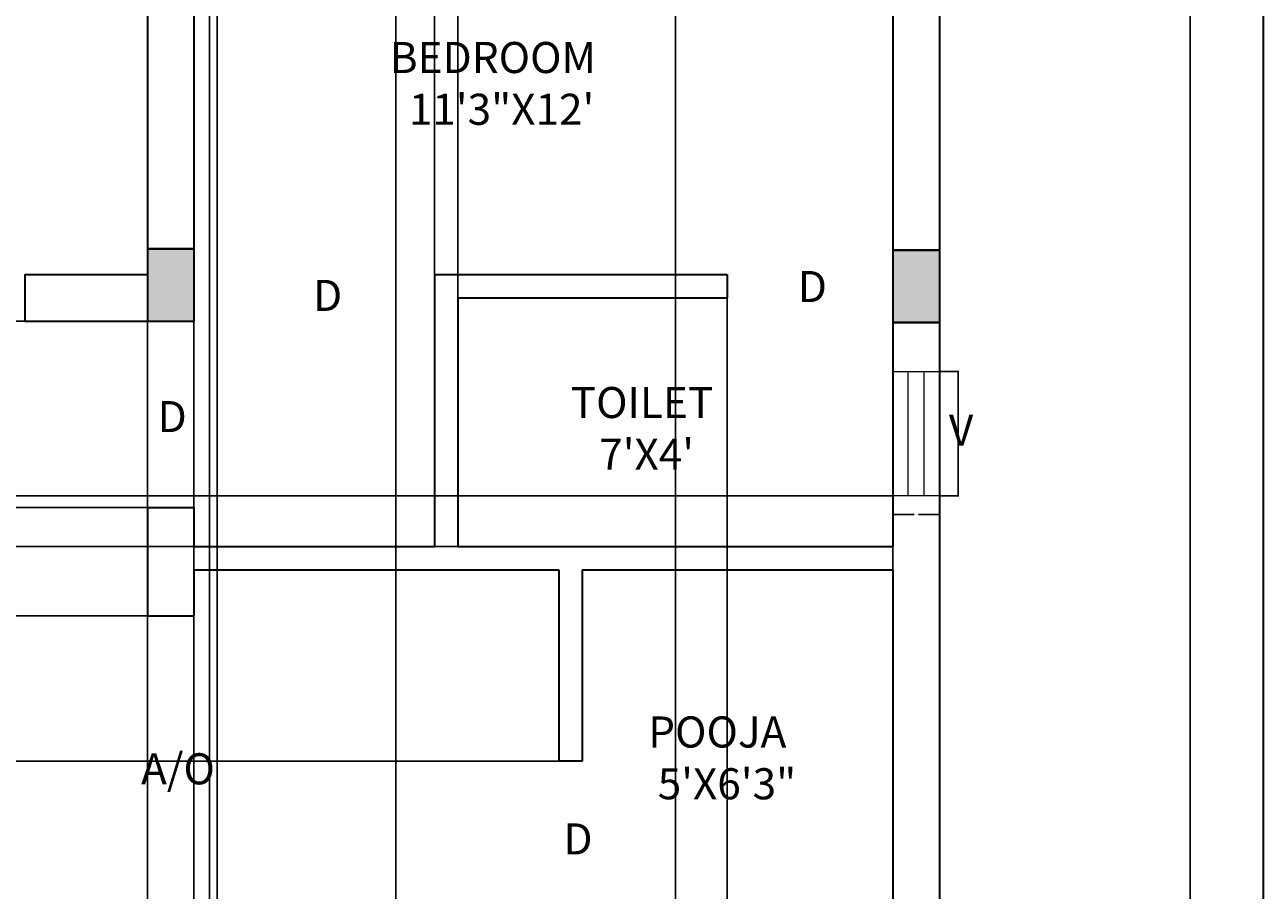
# Model space of a CAD drawing. Units: inches. Extents: x 2243 to 2668, y 14541 to 15226.
# Tile 4 of 5: x 2428 to 2668, y 14904 to 15071. Entities that reach past the tile are written whole.
import ezdxf

# ---------------------------------------------------------------- set-up
doc = ezdxf.new("R2010")
doc.units = ezdxf.units.IN
doc.header["$MEASUREMENT"] = 0
for name, color, linetype, lineweight in [('A-ANNO-DIMS', 2, 'Continuous', 18), ('A-ANNO-SYMB', 3, 'Continuous', 18), ('A-ANNO-TTLB', 7, 'Continuous', 35), ('A-AREA-IDEN', 7, 'Continuous', 18), ('A-COLS', 7, 'Continuous', 40), ('A-COLS-PATT', 7, 'Continuous', 13), ('A-GLAZ-VENT', 4, 'Continuous', 18), ('A-WALL', 7, 'Continuous', 35)]:
    doc.layers.add(name, color=color, linetype=linetype, lineweight=lineweight)
doc.styles.get("Standard").update_dxf_attribs({"font": 'arial.ttf'})
doc.dimstyles.get("Standard").update_dxf_attribs({"dimtxt": 0.18, "dimasz": 0.18, "dimexe": 0.18, "dimexo": 0.0625, "dimgap": 0.09, "dimtad": 0, "dimtih": 1, "dimtoh": 1, "dimdec": 4, "dimzin": 0, "dimdsep": 46, "dimtxsty": 'Standard', "dimcen": 0.09, "dimadec": 0, "dimazin": 0, "dimtfac": 1, "dimtdec": 4, "dimtofl": 0, "dimtmove": 0, "dimatfit": 3, "dimfxl": 1, "dimtolj": 1, "dimtzin": 0, "dimarcsym": 0})

# ---------------------------------------------------------------- blocks, each defined once
blk = doc.blocks.new('VENT-24IN')
for p, q in [((0, 24), (9, 24)), ((0, 0), (0, 24)), ((3, 0), (3, 24)), ((6, 24), (6, 0)), ((9, 24), (9, 0)), ((9, 0), (0, 0))]:
    blk.add_line(p, q)
blk = doc.blocks.new('*D9')
at = {"layer": 'A-ANNO-DIMS', "color": 0, "lineweight": -2, "transparency": 16777216}
for p, q in [((2605.02, 15004.42), (2608.74, 15004.42)), ((2608.56, 15004.24), (2608.56, 14992.6)), ((2608.56, 14980.6), (2608.56, 14992.24)), ((2605.02, 14980.42), (2608.74, 14980.42))]:
    blk.add_line(p, q, dxfattribs=at)
at = {"layer": 'A-ANNO-DIMS', "color": 0, "transparency": 16777216}
for points in [[(2608.53, 15004.24), (2608.59, 15004.24), (2608.56, 15004.42)], [(2608.53, 14980.6), (2608.59, 14980.6), (2608.56, 14980.42)]]:
    blk.add_solid(points, dxfattribs=at)
at = {"layer": 'Defpoints', "color": 0, "transparency": 16777216}
for p in [(2604.96, 15004.42), (2608.56, 15004.42), (2604.96, 14980.42)]:
    blk.add_point(p, dxfattribs=at)
at = {"layer": 'A-ANNO-DIMS', "color": 0, "transparency": 16777216, "insert": (2608.56, 14992.42), "char_height": 0.18, "attachment_point": 5}
blk.add_mtext('\\A1;VENT 24 TYP.', dxfattribs=at)
blk = doc.blocks.new('*D10')
at = {"layer": 'A-ANNO-DIMS', "color": 0, "lineweight": -2, "transparency": 16777216}
for p, q in [((2595.96, 14980.35), (2595.96, 14976.64)), ((2604.96, 14980.35), (2604.96, 14976.64)), ((2596.14, 14976.82), (2600, 14976.82)), ((2604.78, 14976.82), (2600.92, 14976.82))]:
    blk.add_line(p, q, dxfattribs=at)
at = {"layer": 'A-ANNO-DIMS', "color": 0, "transparency": 16777216}
for points in [[(2596.14, 14976.85), (2596.14, 14976.79), (2595.96, 14976.82)], [(2604.78, 14976.85), (2604.78, 14976.79), (2604.96, 14976.82)]]:
    blk.add_solid(points, dxfattribs=at)
at = {"layer": 'Defpoints', "color": 0, "transparency": 16777216}
for p in [(2595.96, 14980.42), (2604.96, 14980.42), (2604.96, 14976.82)]:
    blk.add_point(p, dxfattribs=at)
at = {"layer": 'A-ANNO-DIMS', "color": 0, "transparency": 16777216, "insert": (2600.46, 14976.82), "char_height": 0.18, "attachment_point": 5}
blk.add_mtext('\\A1;9 TYP.', dxfattribs=at)
blk = doc.blocks.new('*D18')
at = {"layer": 'A-ANNO-DIMS', "color": 0, "lineweight": -2, "transparency": 16777216}
for p, q in [((2605.02, 15176.14), (2653.58, 15176.14)), ((2653.4, 15175.96), (2653.4, 14877.07)), ((2653.4, 14577.82), (2653.4, 14876.7)), ((2605.02, 14577.64), (2653.58, 14577.64))]:
    blk.add_line(p, q, dxfattribs=at)
at = {"layer": 'A-ANNO-DIMS', "color": 0, "transparency": 16777216}
for points in [[(2653.37, 15175.96), (2653.43, 15175.96), (2653.4, 15176.14)], [(2653.37, 14577.82), (2653.43, 14577.82), (2653.4, 14577.64)]]:
    blk.add_solid(points, dxfattribs=at)
at = {"layer": 'Defpoints', "color": 0, "transparency": 16777216}
for p in [(2604.96, 15176.14), (2653.4, 15176.14), (2604.96, 14577.64)]:
    blk.add_point(p, dxfattribs=at)
at = {"layer": 'A-ANNO-DIMS', "color": 0, "transparency": 16777216, "insert": (2653.4, 14876.89), "char_height": 0.18, "attachment_point": 5}
blk.add_mtext('\\A1;598.5', dxfattribs=at)
blk = doc.blocks.new('*D31')
at = {"layer": 'A-ANNO-DIMS', "color": 0, "lineweight": -2, "transparency": 16777216}
for p, q in [((2595.9, 14980.42), (2243.57, 14980.42)), ((2243.75, 14980.24), (2243.75, 14975.71)), ((2243.75, 14970.82), (2243.75, 14975.34)), ((2595.9, 14970.64), (2243.57, 14970.64))]:
    blk.add_line(p, q, dxfattribs=at)
at = {"layer": 'A-ANNO-DIMS', "color": 0, "transparency": 16777216}
for points in [[(2243.72, 14980.24), (2243.78, 14980.24), (2243.75, 14980.42)], [(2243.72, 14970.82), (2243.78, 14970.82), (2243.75, 14970.64)]]:
    blk.add_solid(points, dxfattribs=at)
at = {"layer": 'Defpoints', "color": 0, "transparency": 16777216}
for p in [(2243.75, 14980.42), (2595.96, 14980.42), (2595.96, 14970.64)]:
    blk.add_point(p, dxfattribs=at)
at = {"layer": 'A-ANNO-DIMS', "color": 0, "transparency": 16777216, "insert": (2243.75, 14975.53), "char_height": 0.18, "attachment_point": 5}
blk.add_mtext('\\A1;9.78', dxfattribs=at)
blk = doc.blocks.new('*D35')
at = {"layer": 'A-ANNO-DIMS', "color": 0, "lineweight": -2, "transparency": 16777216}
for p, q in [((2411.89, 14673.7), (2411.89, 15225.04)), ((2412.07, 15224.86), (2431.53, 15224.86)), ((2451.78, 15224.86), (2432.32, 15224.86)), ((2451.96, 14673.7), (2451.96, 15225.04))]:
    blk.add_line(p, q, dxfattribs=at)
at = {"layer": 'A-ANNO-DIMS', "color": 0, "transparency": 16777216}
for points in [[(2412.07, 15224.89), (2412.07, 15224.83), (2411.89, 15224.86)], [(2451.78, 15224.89), (2451.78, 15224.83), (2451.96, 15224.86)]]:
    blk.add_solid(points, dxfattribs=at)
at = {"layer": 'Defpoints', "color": 0, "transparency": 16777216}
for p in [(2451.96, 15224.86), (2411.89, 14673.64), (2451.96, 14673.64)]:
    blk.add_point(p, dxfattribs=at)
at = {"layer": 'A-ANNO-DIMS', "color": 0, "transparency": 16777216, "insert": (2431.93, 15224.86), "char_height": 0.18, "attachment_point": 5}
blk.add_mtext('\\A1;40.07', dxfattribs=at)
blk = doc.blocks.new('*D36')
at = {"layer": 'A-ANNO-DIMS', "color": 0, "lineweight": -2, "transparency": 16777216}
for p, q in [((2460.96, 14673.7), (2460.96, 15225.04)), ((2461.14, 15224.86), (2462.95, 15224.86)), ((2465.28, 15224.86), (2463.47, 15224.86)), ((2465.46, 14673.7), (2465.46, 15225.04))]:
    blk.add_line(p, q, dxfattribs=at)
at = {"layer": 'A-ANNO-DIMS', "color": 0, "transparency": 16777216}
for points in [[(2461.14, 15224.89), (2461.14, 15224.83), (2460.96, 15224.86)], [(2465.28, 15224.89), (2465.28, 15224.83), (2465.46, 15224.86)]]:
    blk.add_solid(points, dxfattribs=at)
at = {"layer": 'Defpoints', "color": 0, "transparency": 16777216}
for p in [(2465.46, 15224.86), (2460.96, 14673.64), (2465.46, 14673.64)]:
    blk.add_point(p, dxfattribs=at)
at = {"layer": 'A-ANNO-DIMS', "color": 0, "transparency": 16777216, "insert": (2463.21, 15224.86), "char_height": 0.18, "attachment_point": 5}
blk.add_mtext('\\A1;4.5', dxfattribs=at)
blk = doc.blocks.new('*D37')
at = {"layer": 'A-ANNO-DIMS', "color": 0, "lineweight": -2, "transparency": 16777216}
for p, q in [((2463.96, 14586.7), (2463.96, 15225.04)), ((2464.14, 15224.86), (2508.74, 15224.86)), ((2553.78, 15224.86), (2509.18, 15224.86)), ((2553.96, 14586.7), (2553.96, 15225.04))]:
    blk.add_line(p, q, dxfattribs=at)
at = {"layer": 'A-ANNO-DIMS', "color": 0, "transparency": 16777216}
for points in [[(2464.14, 15224.89), (2464.14, 15224.83), (2463.96, 15224.86)], [(2553.78, 15224.89), (2553.78, 15224.83), (2553.96, 15224.86)]]:
    blk.add_solid(points, dxfattribs=at)
at = {"layer": 'Defpoints', "color": 0, "transparency": 16777216}
for p in [(2553.96, 15224.86), (2463.96, 14586.64), (2553.96, 14586.64)]:
    blk.add_point(p, dxfattribs=at)
at = {"layer": 'A-ANNO-DIMS', "color": 0, "transparency": 16777216, "insert": (2508.96, 15224.86), "char_height": 0.18, "attachment_point": 5}
blk.add_mtext('\\A1;90', dxfattribs=at)
blk = doc.blocks.new('*D48')
at = {"layer": 'A-ANNO-DIMS', "color": 0, "lineweight": -2, "transparency": 16777216}
for p, q in [((2463.96, 14891.2), (2463.96, 15225.04)), ((2464.14, 15224.86), (2481.74, 15224.86)), ((2499.78, 15224.86), (2482.18, 15224.86)), ((2499.96, 14891.2), (2499.96, 15225.04))]:
    blk.add_line(p, q, dxfattribs=at)
at = {"layer": 'A-ANNO-DIMS', "color": 0, "transparency": 16777216}
for points in [[(2464.14, 15224.89), (2464.14, 15224.83), (2463.96, 15224.86)], [(2499.78, 15224.89), (2499.78, 15224.83), (2499.96, 15224.86)]]:
    blk.add_solid(points, dxfattribs=at)
at = {"layer": 'Defpoints', "color": 0, "transparency": 16777216}
for p in [(2499.96, 15224.86), (2463.96, 14891.14), (2499.96, 14891.14)]:
    blk.add_point(p, dxfattribs=at)
at = {"layer": 'A-ANNO-DIMS', "color": 0, "transparency": 16777216, "insert": (2481.96, 15224.86), "char_height": 0.18, "attachment_point": 5}
blk.add_mtext('\\A1;36', dxfattribs=at)
blk = doc.blocks.new('*D49')
at = {"layer": 'A-ANNO-DIMS', "color": 0, "lineweight": -2, "transparency": 16777216}
for p, q in [((2563.96, 15018.57), (2563.96, 14545.86)), ((2595.96, 15013.82), (2595.96, 14545.86)), ((2564.14, 14546.04), (2579.74, 14546.04)), ((2595.78, 14546.04), (2580.18, 14546.04))]:
    blk.add_line(p, q, dxfattribs=at)
at = {"layer": 'A-ANNO-DIMS', "color": 0, "transparency": 16777216}
for points in [[(2564.14, 14546.07), (2564.14, 14546.01), (2563.96, 14546.04)], [(2595.78, 14546.07), (2595.78, 14546.01), (2595.96, 14546.04)]]:
    blk.add_solid(points, dxfattribs=at)
at = {"layer": 'Defpoints', "color": 0, "transparency": 16777216}
for p in [(2563.96, 15018.64), (2595.96, 15013.89), (2595.96, 14546.04)]:
    blk.add_point(p, dxfattribs=at)
at = {"layer": 'A-ANNO-DIMS', "color": 0, "transparency": 16777216, "insert": (2579.96, 14546.04), "char_height": 0.18, "attachment_point": 5}
blk.add_mtext('\\A1;32', dxfattribs=at)
blk = doc.blocks.new('*D51')
at = {"layer": 'A-ANNO-DIMS', "color": 0, "lineweight": -2, "transparency": 16777216}
for p, q in [((2531.4, 14929.14), (2243.57, 14929.14)), ((2243.75, 14928.96), (2243.75, 14913.32)), ((2243.75, 14897.32), (2243.75, 14912.95)), ((2531.4, 14897.14), (2243.57, 14897.14))]:
    blk.add_line(p, q, dxfattribs=at)
at = {"layer": 'A-ANNO-DIMS', "color": 0, "transparency": 16777216}
for points in [[(2243.72, 14928.96), (2243.78, 14928.96), (2243.75, 14929.14)], [(2243.72, 14897.32), (2243.78, 14897.32), (2243.75, 14897.14)]]:
    blk.add_solid(points, dxfattribs=at)
at = {"layer": 'Defpoints', "color": 0, "transparency": 16777216}
for p in [(2243.75, 14929.14), (2531.46, 14929.14), (2531.46, 14897.14)]:
    blk.add_point(p, dxfattribs=at)
at = {"layer": 'A-ANNO-DIMS', "color": 0, "transparency": 16777216, "insert": (2243.75, 14913.14), "char_height": 0.18, "attachment_point": 5}
blk.add_mtext('\\A1;32', dxfattribs=at)
blk = doc.blocks.new('*D52')
at = {"layer": 'A-ANNO-DIMS', "color": 0, "lineweight": -2, "transparency": 16777216}
for p, q in [((2460.96, 15014.2), (2460.96, 15225.04)), ((2461.14, 15224.86), (2483.88, 15224.86)), ((2507.28, 15224.86), (2484.54, 15224.86)), ((2507.46, 15023.2), (2507.46, 15225.04))]:
    blk.add_line(p, q, dxfattribs=at)
at = {"layer": 'A-ANNO-DIMS', "color": 0, "transparency": 16777216}
for points in [[(2461.14, 15224.89), (2461.14, 15224.83), (2460.96, 15224.86)], [(2507.28, 15224.89), (2507.28, 15224.83), (2507.46, 15224.86)]]:
    blk.add_solid(points, dxfattribs=at)
at = {"layer": 'Defpoints', "color": 0, "transparency": 16777216}
for p in [(2507.46, 15224.86), (2507.46, 15023.14), (2460.96, 15014.14)]:
    blk.add_point(p, dxfattribs=at)
at = {"layer": 'A-ANNO-DIMS', "color": 0, "transparency": 16777216, "insert": (2484.21, 15224.86), "char_height": 0.18, "attachment_point": 5}
blk.add_mtext('\\A1;46.5', dxfattribs=at)
blk = doc.blocks.new('*D53')
at = {"layer": 'A-ANNO-DIMS', "color": 0, "lineweight": -2, "transparency": 16777216}
for p, q in [((2451.9, 15014.14), (2243.57, 15014.14)), ((2243.75, 15013.96), (2243.75, 14996.32)), ((2243.75, 14978.32), (2243.75, 14995.95)), ((2451.9, 14978.14), (2243.57, 14978.14))]:
    blk.add_line(p, q, dxfattribs=at)
at = {"layer": 'A-ANNO-DIMS', "color": 0, "transparency": 16777216}
for points in [[(2243.72, 15013.96), (2243.78, 15013.96), (2243.75, 15014.14)], [(2243.72, 14978.32), (2243.78, 14978.32), (2243.75, 14978.14)]]:
    blk.add_solid(points, dxfattribs=at)
at = {"layer": 'Defpoints', "color": 0, "transparency": 16777216}
for p in [(2243.75, 15014.14), (2451.96, 15014.14), (2451.96, 14978.14)]:
    blk.add_point(p, dxfattribs=at)
at = {"layer": 'A-ANNO-DIMS', "color": 0, "transparency": 16777216, "insert": (2243.75, 14996.14), "char_height": 0.18, "attachment_point": 5}
blk.add_mtext('\\A1;36', dxfattribs=at)
blk = doc.blocks.new('*D54')
at = {"layer": 'A-ANNO-DIMS', "color": 0, "lineweight": -2, "transparency": 16777216}
for p, q in [((2451.9, 14957.21), (2243.57, 14957.21)), ((2243.75, 14957.03), (2243.75, 14927.48)), ((2243.75, 14897.56), (2243.75, 14927.11)), ((2451.9, 14897.38), (2243.57, 14897.38))]:
    blk.add_line(p, q, dxfattribs=at)
at = {"layer": 'A-ANNO-DIMS', "color": 0, "transparency": 16777216}
for points in [[(2243.72, 14957.03), (2243.78, 14957.03), (2243.75, 14957.21)], [(2243.72, 14897.56), (2243.78, 14897.56), (2243.75, 14897.38)]]:
    blk.add_solid(points, dxfattribs=at)
at = {"layer": 'Defpoints', "color": 0, "transparency": 16777216}
for p in [(2243.75, 14957.21), (2451.96, 14957.21), (2451.96, 14897.38)]:
    blk.add_point(p, dxfattribs=at)
at = {"layer": 'A-ANNO-DIMS', "color": 0, "transparency": 16777216, "insert": (2243.75, 14927.3), "char_height": 0.18, "attachment_point": 5}
blk.add_mtext('\\A1;59.83', dxfattribs=at)
blk = doc.blocks.new('*D55')
at = {"layer": 'A-ANNO-DIMS', "color": 0, "lineweight": -2, "transparency": 16777216}
for p, q in [((2507.46, 14970.7), (2507.46, 15225.04)), ((2507.64, 15224.86), (2509.45, 15224.86)), ((2511.78, 15224.86), (2509.97, 15224.86)), ((2511.96, 14970.7), (2511.96, 15225.04))]:
    blk.add_line(p, q, dxfattribs=at)
at = {"layer": 'A-ANNO-DIMS', "color": 0, "transparency": 16777216}
for points in [[(2507.64, 15224.89), (2507.64, 15224.83), (2507.46, 15224.86)], [(2511.78, 15224.89), (2511.78, 15224.83), (2511.96, 15224.86)]]:
    blk.add_solid(points, dxfattribs=at)
at = {"layer": 'Defpoints', "color": 0, "transparency": 16777216}
for p in [(2507.46, 15224.86), (2507.46, 14970.64), (2511.96, 14970.64)]:
    blk.add_point(p, dxfattribs=at)
at = {"layer": 'A-ANNO-DIMS', "color": 0, "transparency": 16777216, "insert": (2509.71, 15224.86), "char_height": 0.18, "attachment_point": 5}
blk.add_mtext('\\A1;4.5', dxfattribs=at)

msp = doc.modelspace()

# ---------------------------------------------------------------- hatches: boundary and pattern name
at = {"layer": 'A-COLS-PATT'}
h = msp.add_hatch(color=256, dxfattribs=at)
h.dxf.hatch_style = 1
h.paths.add_polyline_path([(2301.96, 15176.1368), (2292.96, 15176.1368), (2292.96, 15162.1368), (2301.96, 15162.1368)])
h.paths.add_polyline_path([(2460.96, 15176.1368), (2451.96, 15176.1368), (2451.96, 15162.1368), (2460.96, 15162.1368)])
h.paths.add_polyline_path([(2604.96, 15176.1368), (2595.96, 15176.1368), (2595.96, 15162.1368), (2604.96, 15162.1368)])
h.paths.add_polyline_path([(2301.96, 15028.1368), (2292.96, 15028.1368), (2292.96, 15014.1368), (2301.96, 15014.1368)])
h.paths.add_polyline_path([(2460.96, 15028.1368), (2451.96, 15028.1368), (2451.96, 15014.1368), (2460.96, 15014.1368)])
h.paths.add_polyline_path([(2604.96, 15027.8868), (2595.96, 15027.8868), (2595.96, 15013.8868), (2604.96, 15013.8868)])
h.paths.add_polyline_path([(2301.96, 14891.1368), (2292.96, 14891.1368), (2292.96, 14877.1368), (2301.96, 14877.1368)])
h.paths.add_polyline_path([(2460.96, 14891.1368), (2451.96, 14891.1368), (2451.96, 14877.1368), (2460.96, 14877.1368)])
h.paths.add_polyline_path([(2604.96, 14891.1368), (2595.96, 14891.1368), (2595.96, 14877.1368), (2604.96, 14877.1368)])
h.paths.add_polyline_path([(2301.96, 14678.6368), (2292.96, 14678.6368), (2292.96, 14664.6368), (2301.96, 14664.6368)])
h.paths.add_polyline_path([(2460.96, 14678.6368), (2451.96, 14678.6368), (2451.96, 14664.6368), (2460.96, 14664.6368)])
h.paths.add_polyline_path([(2604.96, 14678.6368), (2595.96, 14678.6368), (2595.96, 14664.6368), (2604.96, 14664.6368)])
h.paths.add_polyline_path([(2604.96, 14591.6368), (2595.96, 14591.6368), (2595.96, 14577.6368), (2604.96, 14577.6368)])
h.paths.add_polyline_path([(2460.96, 14591.6368), (2451.96, 14591.6368), (2451.96, 14577.6368), (2460.96, 14577.6368)])
h.paths.add_polyline_path([(2306.96, 14586.6368), (2292.96, 14586.6368), (2292.96, 14577.6368), (2306.96, 14577.6368)])

# ---------------------------------------------------------------- linework, layer by layer
at = {"layer": 'A-ANNO-TTLB'}
msp.add_lwpolyline([(2246.1122, 15225.9536), (2667.5226, 15225.9536), (2667.5226, 14540.814), (2246.1122, 14540.814)], close=True, dxfattribs=at)
at = {"layer": 'A-COLS'}
for p, q in [((2451.96, 15028.1368), (2460.96, 15028.1368)), ((2595.96, 15027.8868), (2604.96, 15027.8868)), ((2604.96, 15013.8868), (2595.96, 15013.8868))]:
    msp.add_line(p, q, dxfattribs=at)
at = {"layer": 'A-WALL'}
for p, q in [((2451.96, 15176.1368), (2451.96, 15014.1368)), ((2460.96, 15176.1368), (2460.96, 15014.1368)), ((2595.96, 15176.1368), (2595.96, 14970.6368)), ((2604.96, 15176.1368), (2604.96, 14577.6368)), ((2428.2818, 15023.1368), (2428.2818, 15014.1368)), ((2428.2818, 15023.1368), (2451.96, 15023.1368)), ((2507.46, 15023.1368), (2507.46, 14970.6368)), ((2507.46, 15023.1368), (2563.96, 15023.1368)), ((2563.96, 15023.1368), (2563.96, 15018.6368)), ((2511.96, 15018.6368), (2563.96, 15018.6368)), ((2511.96, 15018.6368), (2511.96, 14970.6368)), ((2428.2818, 15014.1368), (2460.96, 15014.1368)), ((2451.96, 14978.1368), (2460.96, 14978.1368)), ((2451.96, 14978.1368), (2451.96, 14957.2115)), ((2460.96, 14978.1368), (2460.96, 14970.6368)), ((2460.96, 14970.6368), (2507.46, 14970.6368)), ((2511.96, 14970.6368), (2595.96, 14970.6368)), ((2460.96, 14966.1368), (2531.46, 14966.1368)), ((2460.96, 14966.1368), (2460.96, 14957.2115)), ((2531.46, 14966.1368), (2531.46, 14929.1368)), ((2535.96, 14966.1368), (2535.96, 14929.1368)), ((2535.96, 14966.1368), (2595.96, 14966.1368)), ((2595.96, 14966.1368), (2595.96, 14726.1368)), ((2451.96, 14957.2115), (2460.96, 14957.2115)), ((2535.96, 14929.1368), (2531.46, 14929.1368))]:
    msp.add_line(p, q, dxfattribs=at)

# ---------------------------------------------------------------- block references
at = {"layer": 'A-GLAZ-VENT'}
msp.add_blockref('VENT-24IN', (2595.96, 14980.416), dxfattribs=at)

# ---------------------------------------------------------------- texts
at = {"layer": 'A-ANNO-SYMB', "char_height": 6, "attachment_point": 1}
for s, width, insert in [('D', 14.74723, (2483.9696, 15022.1243)), ('D', 14.74723, (2577.6086, 15023.8409)), ('D', 14.74723, (2453.9437, 14998.7205)), ('V', 9.339447, (2606.8045, 14996.0843)), ('A/O', 16.844499, (2450.7538, 14930.6881)), ('D', 14.74723, (2532.3326, 14917.1436))]:
    msp.add_mtext_dynamic_manual_height_columns(s, width=width, gutter_width=30, heights=[0], dxfattribs=dict(at, insert=insert))
at = {"layer": 'A-AREA-IDEN', "char_height": 6, "attachment_point": 1}
for s, width, insert in [('BEDROOM\\P  11\'3"X12\'', 68.414562, (2498.7991, 15068.08)), ("TOILET\\P   7'X4'", 37.402675, (2533.7464, 15001.4384)), (' POOJA\\P  5\'X6\'3"', 39.732507, (2546.886, 14937.799))]:
    msp.add_mtext_dynamic_manual_height_columns(s, width=width, gutter_width=30, heights=[0], dxfattribs=dict(at, insert=insert))

# ---------------------------------------------------------------- dimensions: what is measured, and where the dimension line sits
at = {"layer": 'A-ANNO-DIMS'}
for base, p1, p2, override, picture, middle in [((2451.96, 15224.8619), (2411.8914, 14673.6368), (2451.96, 14673.6368), {"dimdec": 2, "dimlfac": 1, "dimrnd": 0, "dimzin": 0, "dimdsep": 46, "dimlunit": 2}, '*D35', (2431.9257, 15224.8619)), ((2465.46, 15224.8619), (2460.96, 14673.6368), (2465.46, 14673.6368), {"dimdec": 1, "dimlfac": 1, "dimrnd": 0, "dimzin": 0, "dimdsep": 46, "dimlunit": 2}, '*D36', (2463.21, 15224.8619)), ((2507.46, 15224.8619), (2460.96, 15014.1368), (2507.46, 15023.1368), {"dimdec": 1, "dimlfac": 1, "dimrnd": 0, "dimzin": 0, "dimdsep": 46, "dimlunit": 2}, '*D52', (2484.21, 15224.8619)), ((2553.96, 15224.8619), (2463.96, 14586.6368), (2553.96, 14586.6368), {"dimdec": 0, "dimlfac": 1, "dimrnd": 0, "dimzin": 0, "dimdsep": 46, "dimlunit": 2}, '*D37', (2508.96, 15224.8619)), ((2499.96, 15224.8619), (2463.96, 14891.1368), (2499.96, 14891.1368), {"dimdec": 0, "dimlfac": 1, "dimrnd": 0, "dimzin": 0, "dimdsep": 46, "dimlunit": 2}, '*D48', (2481.96, 15224.8619)), ((2507.46, 15224.8619), (2511.96, 14970.6368), (2507.46, 14970.6368), {"dimdec": 1, "dimlfac": 1, "dimrnd": 0, "dimzin": 0, "dimdsep": 46, "dimlunit": 2}, '*D55', (2509.71, 15224.8619)), ((2595.96, 14546.0368), (2563.96, 15018.6368), (2595.96, 15013.8868), {"dimdec": 0, "dimlfac": 1, "dimrnd": 0, "dimzin": 0, "dimdsep": 46, "dimlunit": 2}, '*D49', (2579.96, 14546.0368))]:
    dim = msp.add_linear_dim(base=base, p1=p1, p2=p2, dimstyle='Standard', override=override, dxfattribs=at)
    dim.commit()
    dim.dimension.update_dxf_attribs({"geometry": picture, "text_midpoint": middle})
for base, p1, p2, override, picture, middle in [((2653.4036, 15176.1368), (2604.96, 14577.6368), (2604.96, 15176.1368), {"dimdec": 1, "dimlfac": 1, "dimrnd": 0, "dimzin": 0, "dimdsep": 46, "dimlunit": 2}, '*D18', (2653.4036, 14876.8868)), ((2243.7531, 15014.1368), (2451.96, 14978.1368), (2451.96, 15014.1368), {"dimdec": 0, "dimlfac": 1, "dimrnd": 0, "dimzin": 0, "dimdsep": 46, "dimlunit": 2}, '*D53', (2243.7531, 14996.1368)), ((2243.7531, 14980.4164), (2595.96, 14970.6368), (2595.96, 14980.4164), {"dimdec": 2, "dimlfac": 1, "dimrnd": 0, "dimzin": 0, "dimdsep": 46, "dimlunit": 2}, '*D31', (2243.7531, 14975.5266)), ((2243.7531, 14957.2115), (2451.96, 14897.3823), (2451.96, 14957.2115), {"dimdec": 2, "dimlfac": 1, "dimrnd": 0, "dimzin": 0, "dimdsep": 46, "dimlunit": 2}, '*D54', (2243.7531, 14927.2969)), ((2243.7531, 14929.1368), (2531.46, 14897.1368), (2531.46, 14929.1368), {"dimdec": 0, "dimlfac": 1, "dimrnd": 0, "dimzin": 0, "dimdsep": 46, "dimlunit": 2}, '*D51', (2243.7531, 14913.1368))]:
    dim = msp.add_linear_dim(base=base, p1=p1, p2=p2, angle=90, dimstyle='Standard', override=override, dxfattribs=at)
    dim.commit()
    dim.dimension.update_dxf_attribs({"geometry": picture, "text_midpoint": middle})
dim = msp.add_linear_dim(base=(2608.56, 15004.4164), p1=(2604.96, 14980.4164), p2=(2604.96, 15004.4164), angle=90, text='VENT <> TYP.', dimstyle='Standard', override={"dimdec": 0, "dimlfac": 1, "dimrnd": 0, "dimzin": 0, "dimdsep": 46, "dimlunit": 2}, dxfattribs=at)
dim.commit()
dim.dimension.update_dxf_attribs({"geometry": '*D9', "text_midpoint": (2608.56, 14992.4164)})
dim = msp.add_linear_dim(base=(2604.96, 14976.8164), p1=(2595.96, 14980.4164), p2=(2604.96, 14980.4164), text='<> TYP.', dimstyle='Standard', override={"dimdec": 0, "dimlfac": 1, "dimrnd": 0, "dimzin": 0, "dimdsep": 46, "dimlunit": 2}, dxfattribs=at)
dim.commit()
dim.dimension.update_dxf_attribs({"geometry": '*D10', "text_midpoint": (2600.46, 14976.8164)})

doc.saveas('drawing.dxf')
